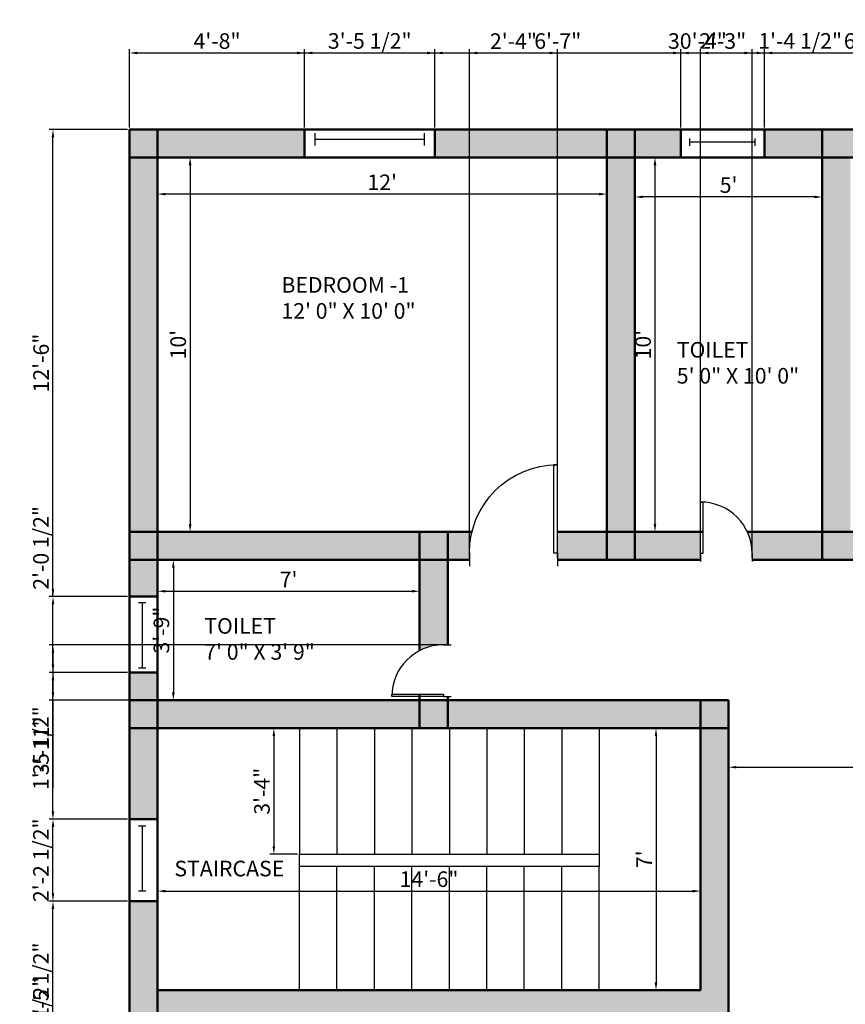
# Model space of a CAD drawing. Units: millimetres. Extents: x 2784 to 3697, y 603 to 1406.
# Tile 9 of 10: x 3272 to 3537, y 953 to 1268. Entities that reach past the tile are written whole.
import ezdxf

# ---------------------------------------------------------------- set-up
doc = ezdxf.new("R2010")
doc.units = ezdxf.units.MM
for name, color, linetype, lineweight in [('A-ANNO-DIMS', 140, 'Continuous', 18), ('A-AREA-IDEN', 150, 'Continuous', 25), ('A-DOOR', 10, 'Continuous', 25), ('A-FLOR-STRS', 200, 'Continuous', 25), ('A-GLAZ', 30, 'Continuous', 25), ('A-WALL', 2, 'Continuous', 50), ('A-WALL-PATT', 8, 'Continuous', 13)]:
    doc.layers.add(name, color=color, linetype=linetype, lineweight=lineweight)
doc.styles.get("Standard").update_dxf_attribs({"font": 'arial.ttf'})
doc.dimstyles.new('ISO-25', dxfattribs={"dimtxt": 5, "dimasz": 2.5, "dimexe": 1.25, "dimexo": 0.625, "dimtad": 1, "dimdec": 0, "dimlunit": 3, "dimtxsty": 'Standard', "dimcen": 2.5, "dimadec": 0, "dimazin": 0, "dimtfac": 1, "dimtdec": 0, "dimtmove": 0, "dimatfit": 3, "dimfxl": 1, "dimarcsym": 0})

# ---------------------------------------------------------------- blocks, each defined once
blk = doc.blocks.new('*U2')
for p, q in [((0, 0), (0, -6)), ((40, 0), (40, -6))]:
    blk.add_line(p, q)
blk.add_lwpolyline([(0, 0), (0, 40), (1.75, 40), (1.75, 0)], close=True)
blk.add_arc((0, 0), 40, 0, 90)
blk = doc.blocks.new('*U38')
for p, q in [((0, 4), (0, 0)), ((36, 4), (36, 0)), ((0, 2), (36, 2))]:
    blk.add_line(p, q)
blk = doc.blocks.new('*D39')
at = {"layer": 'A-ANNO-DIMS', "color": 0, "lineweight": -2, "transparency": 16777216}
for p, q in [((3326.67, 1221.78), (3326.67, 1106.78)), ((3327.3, 1224.28), (3327.92, 1224.28)), ((3327.3, 1104.28), (3327.92, 1104.28))]:
    blk.add_line(p, q, dxfattribs=at)
at = {"layer": 'A-ANNO-DIMS', "color": 0, "transparency": 16777216}
for points in [[(3326.25, 1221.78), (3327.09, 1221.78), (3326.67, 1224.28)], [(3326.25, 1106.78), (3327.09, 1106.78), (3326.67, 1104.28)]]:
    blk.add_solid(points, dxfattribs=at)
at = {"layer": 'Defpoints', "color": 0, "transparency": 16777216}
for p in [(3326.67, 1224.28), (3326.67, 1104.28), (3326.67, 1104.28)]:
    blk.add_point(p, dxfattribs=at)
at = {"layer": 'A-ANNO-DIMS', "color": 0, "transparency": 16777216, "insert": (3323.49, 1164.28), "char_height": 5, "attachment_point": 5, "rotation": 90}
blk.add_mtext("10'", dxfattribs=at)
blk = doc.blocks.new('*D40')
at = {"layer": 'A-ANNO-DIMS', "color": 0, "lineweight": -2, "transparency": 16777216}
for p, q in [((3316.23, 1213.16), (3316.23, 1213.79)), ((3457.73, 1212.54), (3318.73, 1212.54)), ((3460.23, 1213.16), (3460.23, 1213.79))]:
    blk.add_line(p, q, dxfattribs=at)
at = {"layer": 'A-ANNO-DIMS', "color": 0, "transparency": 16777216}
for points in [[(3318.73, 1212.95), (3318.73, 1212.12), (3316.23, 1212.54)], [(3457.73, 1212.95), (3457.73, 1212.12), (3460.23, 1212.54)]]:
    blk.add_solid(points, dxfattribs=at)
at = {"layer": 'Defpoints', "color": 0, "transparency": 16777216}
for p in [(3316.23, 1212.54), (3316.23, 1212.54), (3460.23, 1212.54)]:
    blk.add_point(p, dxfattribs=at)
at = {"layer": 'A-ANNO-DIMS', "color": 0, "transparency": 16777216, "insert": (3388.23, 1215.67), "char_height": 5, "attachment_point": 5}
blk.add_mtext("12'", dxfattribs=at)
blk = doc.blocks.new('*D41')
at = {"layer": 'A-ANNO-DIMS', "color": 0, "lineweight": -2, "transparency": 16777216}
for p, q in [((3475.35, 1224.28), (3476.89, 1224.28)), ((3475.64, 1221.78), (3475.64, 1106.78)), ((3475.35, 1104.28), (3476.89, 1104.28))]:
    blk.add_line(p, q, dxfattribs=at)
at = {"layer": 'A-ANNO-DIMS', "color": 0, "transparency": 16777216}
for points in [[(3475.22, 1221.78), (3476.06, 1221.78), (3475.64, 1224.28)], [(3475.22, 1106.78), (3476.06, 1106.78), (3475.64, 1104.28)]]:
    blk.add_solid(points, dxfattribs=at)
at = {"layer": 'Defpoints', "color": 0, "transparency": 16777216}
for p in [(3474.73, 1224.28), (3474.73, 1104.28), (3475.64, 1104.28)]:
    blk.add_point(p, dxfattribs=at)
at = {"layer": 'A-ANNO-DIMS', "color": 0, "transparency": 16777216, "insert": (3472.46, 1164.28), "char_height": 5, "attachment_point": 5, "rotation": 90}
blk.add_mtext("10'", dxfattribs=at)
blk = doc.blocks.new('*D42')
at = {"layer": 'A-ANNO-DIMS', "color": 0, "lineweight": -2, "transparency": 16777216}
for p, q in [((3469.23, 1215.87), (3469.23, 1210.37)), ((3529.23, 1215.87), (3529.23, 1210.37)), ((3526.73, 1211.62), (3471.73, 1211.62))]:
    blk.add_line(p, q, dxfattribs=at)
at = {"layer": 'A-ANNO-DIMS', "color": 0, "transparency": 16777216}
for points in [[(3471.73, 1212.04), (3471.73, 1211.21), (3469.23, 1211.62)], [(3526.73, 1212.04), (3526.73, 1211.21), (3529.23, 1211.62)]]:
    blk.add_solid(points, dxfattribs=at)
at = {"layer": 'Defpoints', "color": 0, "transparency": 16777216}
for p in [(3469.23, 1216.49), (3529.23, 1216.49), (3469.23, 1211.62)]:
    blk.add_point(p, dxfattribs=at)
at = {"layer": 'A-ANNO-DIMS', "color": 0, "transparency": 16777216, "insert": (3499.23, 1214.79), "char_height": 5, "attachment_point": 5}
blk.add_mtext("5'", dxfattribs=at)
blk = doc.blocks.new('*D45')
at = {"layer": 'A-ANNO-DIMS', "color": 0, "lineweight": -2, "transparency": 16777216}
for p, q in [((3321.44, 1095.28), (3322.55, 1095.28)), ((3321.3, 1092.78), (3321.3, 1052.78)), ((3321.44, 1050.28), (3322.55, 1050.28))]:
    blk.add_line(p, q, dxfattribs=at)
at = {"layer": 'A-ANNO-DIMS', "color": 0, "transparency": 16777216}
for points in [[(3320.88, 1092.78), (3321.71, 1092.78), (3321.3, 1095.28)], [(3320.88, 1052.78), (3321.71, 1052.78), (3321.3, 1050.28)]]:
    blk.add_solid(points, dxfattribs=at)
at = {"layer": 'Defpoints', "color": 0, "transparency": 16777216}
for p in [(3320.81, 1095.28), (3320.81, 1050.28), (3321.3, 1050.28)]:
    blk.add_point(p, dxfattribs=at)
at = {"layer": 'A-ANNO-DIMS', "color": 0, "transparency": 16777216, "insert": (3318.12, 1072.78), "char_height": 5, "attachment_point": 5, "rotation": 90}
blk.add_mtext('3\'-9"', dxfattribs=at)
blk = doc.blocks.new('*D46')
at = {"layer": 'A-ANNO-DIMS', "color": 0, "lineweight": -2, "transparency": 16777216}
for p, q in [((3316.23, 1086.57), (3316.23, 1083.98)), ((3400.23, 1085.85), (3400.23, 1086.48)), ((3318.73, 1085.23), (3397.73, 1085.23))]:
    blk.add_line(p, q, dxfattribs=at)
at = {"layer": 'A-ANNO-DIMS', "color": 0, "transparency": 16777216}
for points in [[(3318.73, 1085.64), (3318.73, 1084.81), (3316.23, 1085.23)], [(3397.73, 1085.64), (3397.73, 1084.81), (3400.23, 1085.23)]]:
    blk.add_solid(points, dxfattribs=at)
at = {"layer": 'Defpoints', "color": 0, "transparency": 16777216}
for p in [(3316.23, 1087.2), (3400.23, 1085.23), (3400.23, 1085.23)]:
    blk.add_point(p, dxfattribs=at)
at = {"layer": 'A-ANNO-DIMS', "color": 0, "transparency": 16777216, "insert": (3358.23, 1088.35), "char_height": 5, "attachment_point": 5}
blk.add_mtext("7'", dxfattribs=at)
blk = doc.blocks.new('*D55')
at = {"layer": 'A-ANNO-DIMS', "color": 0, "lineweight": -2, "transparency": 16777216}
for p, q in [((3361.11, 1041.28), (3352.26, 1041.28)), ((3353.51, 1038.78), (3353.51, 1003.45)), ((3361.11, 1000.95), (3352.26, 1000.95))]:
    blk.add_line(p, q, dxfattribs=at)
at = {"layer": 'A-ANNO-DIMS', "color": 0, "transparency": 16777216}
for points in [[(3353.09, 1038.78), (3353.93, 1038.78), (3353.51, 1041.28)], [(3353.09, 1003.45), (3353.93, 1003.45), (3353.51, 1000.95)]]:
    blk.add_solid(points, dxfattribs=at)
at = {"layer": 'Defpoints', "color": 0, "transparency": 16777216}
for p in [(3361.74, 1041.28), (3353.51, 1000.95), (3361.74, 1000.95)]:
    blk.add_point(p, dxfattribs=at)
at = {"layer": 'A-ANNO-DIMS', "color": 0, "transparency": 16777216, "insert": (3350.33, 1021.12), "char_height": 5, "attachment_point": 5, "rotation": 90}
blk.add_mtext('3\'-4"', dxfattribs=at)
blk = doc.blocks.new('*D56')
at = {"layer": 'A-ANNO-DIMS', "color": 0, "lineweight": -2, "transparency": 16777216}
for p, q in [((3316.23, 992.49), (3316.23, 987.85)), ((3490.23, 992.49), (3490.23, 987.85)), ((3318.73, 989.1), (3487.73, 989.1))]:
    blk.add_line(p, q, dxfattribs=at)
at = {"layer": 'A-ANNO-DIMS', "color": 0, "transparency": 16777216}
for points in [[(3318.73, 989.51), (3318.73, 988.68), (3316.23, 989.1)], [(3487.73, 989.51), (3487.73, 988.68), (3490.23, 989.1)]]:
    blk.add_solid(points, dxfattribs=at)
at = {"layer": 'Defpoints', "color": 0, "transparency": 16777216}
for p in [(3316.23, 993.11), (3490.23, 993.11), (3490.23, 989.1)]:
    blk.add_point(p, dxfattribs=at)
at = {"layer": 'A-ANNO-DIMS', "color": 0, "transparency": 16777216, "insert": (3403.23, 992.28), "char_height": 5, "attachment_point": 5}
blk.add_mtext('14\'-6"', dxfattribs=at)
blk = doc.blocks.new('*D57')
at = {"layer": 'A-ANNO-DIMS', "color": 0, "lineweight": -2, "transparency": 16777216}
for p, q in [((3475.97, 1038.78), (3475.97, 959.81)), ((3476.59, 1041.28), (3477.22, 1041.28)), ((3476.59, 957.31), (3477.22, 957.31))]:
    blk.add_line(p, q, dxfattribs=at)
at = {"layer": 'A-ANNO-DIMS', "color": 0, "transparency": 16777216}
for points in [[(3475.55, 1038.78), (3476.38, 1038.78), (3475.97, 1041.28)], [(3475.55, 959.81), (3476.38, 959.81), (3475.97, 957.31)]]:
    blk.add_solid(points, dxfattribs=at)
at = {"layer": 'Defpoints', "color": 0, "transparency": 16777216}
for p in [(3475.97, 1041.28), (3475.97, 957.31), (3475.97, 957.31)]:
    blk.add_point(p, dxfattribs=at)
at = {"layer": 'A-ANNO-DIMS', "color": 0, "transparency": 16777216, "insert": (3472.84, 999.3), "char_height": 5, "attachment_point": 5, "rotation": 90}
blk.add_mtext("7'", dxfattribs=at)
blk = doc.blocks.new('*D59')
at = {"layer": 'A-ANNO-DIMS', "color": 0, "lineweight": -2, "transparency": 16777216}
for p, q in [((3499.23, 1028.23), (3499.23, 1030.07)), ((3662.23, 1028.23), (3662.23, 1030.07)), ((3501.73, 1028.82), (3659.73, 1028.82))]:
    blk.add_line(p, q, dxfattribs=at)
at = {"layer": 'A-ANNO-DIMS', "color": 0, "transparency": 16777216}
for points in [[(3501.73, 1029.23), (3501.73, 1028.4), (3499.23, 1028.82)], [(3659.73, 1029.23), (3659.73, 1028.4), (3662.23, 1028.82)]]:
    blk.add_solid(points, dxfattribs=at)
at = {"layer": 'Defpoints', "color": 0, "transparency": 16777216}
for p in [(3499.23, 1027.6), (3662.23, 1028.82), (3662.23, 1027.6)]:
    blk.add_point(p, dxfattribs=at)
at = {"layer": 'A-ANNO-DIMS', "color": 0, "transparency": 16777216, "insert": (3580.73, 1032), "char_height": 5, "attachment_point": 5}
blk.add_mtext('13\'-7"', dxfattribs=at)
blk = doc.blocks.new('*D110')
at = {"layer": 'A-ANNO-DIMS', "color": 0, "lineweight": -2, "transparency": 16777216}
for p, q in [((3307.23, 1233.91), (3307.23, 1259.03)), ((3309.73, 1257.78), (3668.73, 1257.78)), ((3671.23, 1233.91), (3671.23, 1259.03))]:
    blk.add_line(p, q, dxfattribs=at)
at = {"layer": 'A-ANNO-DIMS', "color": 0, "transparency": 16777216}
for points in [[(3309.73, 1258.2), (3309.73, 1257.36), (3307.23, 1257.78)], [(3668.73, 1258.2), (3668.73, 1257.36), (3671.23, 1257.78)]]:
    blk.add_solid(points, dxfattribs=at)
at = {"layer": 'Defpoints', "color": 0, "transparency": 16777216}
for p in [(3671.23, 1257.78), (3307.23, 1233.28), (3671.23, 1233.28)]:
    blk.add_point(p, dxfattribs=at)
at = {"layer": 'A-ANNO-DIMS', "color": 0, "transparency": 16777216, "insert": (3489.23, 1260.96), "char_height": 5, "attachment_point": 5}
blk.add_mtext('30\'-4"', dxfattribs=at)
blk = doc.blocks.new('*D111')
at = {"layer": 'A-ANNO-DIMS', "color": 0, "lineweight": -2, "transparency": 16777216}
for p, q in [((3307.23, 1233.91), (3307.23, 1259.03)), ((3309.73, 1257.78), (3360.87, 1257.78)), ((3363.37, 1233.91), (3363.37, 1259.03))]:
    blk.add_line(p, q, dxfattribs=at)
at = {"layer": 'A-ANNO-DIMS', "color": 0, "transparency": 16777216}
for points in [[(3309.73, 1258.2), (3309.73, 1257.36), (3307.23, 1257.78)], [(3360.87, 1258.2), (3360.87, 1257.36), (3363.37, 1257.78)]]:
    blk.add_solid(points, dxfattribs=at)
at = {"layer": 'Defpoints', "color": 0, "transparency": 16777216}
for p in [(3363.37, 1257.78), (3307.23, 1233.28), (3363.37, 1233.28)]:
    blk.add_point(p, dxfattribs=at)
at = {"layer": 'A-ANNO-DIMS', "color": 0, "transparency": 16777216, "insert": (3335.3, 1260.96), "char_height": 5, "attachment_point": 5}
blk.add_mtext('4\'-8"', dxfattribs=at)
blk = doc.blocks.new('*D112')
at = {"layer": 'A-ANNO-DIMS', "color": 0, "lineweight": -2, "transparency": 16777216}
for p, q in [((3363.37, 1233.91), (3363.37, 1259.03)), ((3365.87, 1257.78), (3402.6, 1257.78)), ((3405.1, 1233.91), (3405.1, 1259.03))]:
    blk.add_line(p, q, dxfattribs=at)
at = {"layer": 'A-ANNO-DIMS', "color": 0, "transparency": 16777216}
for points in [[(3365.87, 1258.2), (3365.87, 1257.36), (3363.37, 1257.78)], [(3402.6, 1258.2), (3402.6, 1257.36), (3405.1, 1257.78)]]:
    blk.add_solid(points, dxfattribs=at)
at = {"layer": 'Defpoints', "color": 0, "transparency": 16777216}
for p in [(3405.1, 1257.78), (3363.37, 1233.28), (3405.1, 1233.28)]:
    blk.add_point(p, dxfattribs=at)
at = {"layer": 'A-ANNO-DIMS', "color": 0, "transparency": 16777216, "insert": (3384.23, 1260.99), "char_height": 5, "attachment_point": 5}
blk.add_mtext('3\'-5 1/2"', dxfattribs=at)
blk = doc.blocks.new('*D113')
at = {"layer": 'A-ANNO-DIMS', "color": 0, "lineweight": -2, "transparency": 16777216}
for p, q in [((3405.1, 1233.91), (3405.1, 1259.03)), ((3407.6, 1257.78), (3481.39, 1257.78)), ((3483.89, 1233.91), (3483.89, 1259.03))]:
    blk.add_line(p, q, dxfattribs=at)
at = {"layer": 'A-ANNO-DIMS', "color": 0, "transparency": 16777216}
for points in [[(3407.6, 1258.2), (3407.6, 1257.36), (3405.1, 1257.78)], [(3481.39, 1258.2), (3481.39, 1257.36), (3483.89, 1257.78)]]:
    blk.add_solid(points, dxfattribs=at)
at = {"layer": 'Defpoints', "color": 0, "transparency": 16777216}
for p in [(3483.89, 1257.78), (3405.1, 1233.28), (3483.89, 1233.28)]:
    blk.add_point(p, dxfattribs=at)
at = {"layer": 'A-ANNO-DIMS', "color": 0, "transparency": 16777216, "insert": (3444.49, 1260.96), "char_height": 5, "attachment_point": 5}
blk.add_mtext('6\'-7"', dxfattribs=at)
blk = doc.blocks.new('*D114')
at = {"layer": 'A-ANNO-DIMS', "color": 0, "lineweight": -2, "transparency": 16777216}
for p, q in [((3483.89, 1233.91), (3483.89, 1259.03)), ((3486.39, 1257.78), (3508.27, 1257.78)), ((3510.77, 1233.91), (3510.77, 1259.03))]:
    blk.add_line(p, q, dxfattribs=at)
at = {"layer": 'A-ANNO-DIMS', "color": 0, "transparency": 16777216}
for points in [[(3486.39, 1258.2), (3486.39, 1257.36), (3483.89, 1257.78)], [(3508.27, 1258.2), (3508.27, 1257.36), (3510.77, 1257.78)]]:
    blk.add_solid(points, dxfattribs=at)
at = {"layer": 'Defpoints', "color": 0, "transparency": 16777216}
for p in [(3510.77, 1257.78), (3483.89, 1233.28), (3510.77, 1233.28)]:
    blk.add_point(p, dxfattribs=at)
at = {"layer": 'A-ANNO-DIMS', "color": 0, "transparency": 16777216, "insert": (3497.33, 1260.96), "char_height": 5, "attachment_point": 5}
blk.add_mtext('2\'-3"', dxfattribs=at)
blk = doc.blocks.new('*D115')
at = {"layer": 'A-ANNO-DIMS', "color": 0, "lineweight": -2, "transparency": 16777216}
for p, q in [((3510.77, 1233.91), (3510.77, 1259.03)), ((3513.27, 1257.78), (3585.87, 1257.78)), ((3588.37, 1233.91), (3588.37, 1259.03))]:
    blk.add_line(p, q, dxfattribs=at)
at = {"layer": 'A-ANNO-DIMS', "color": 0, "transparency": 16777216}
for points in [[(3513.27, 1258.2), (3513.27, 1257.36), (3510.77, 1257.78)], [(3585.87, 1258.2), (3585.87, 1257.36), (3588.37, 1257.78)]]:
    blk.add_solid(points, dxfattribs=at)
at = {"layer": 'Defpoints', "color": 0, "transparency": 16777216}
for p in [(3588.37, 1257.78), (3510.77, 1233.28), (3588.37, 1233.28)]:
    blk.add_point(p, dxfattribs=at)
at = {"layer": 'A-ANNO-DIMS', "color": 0, "transparency": 16777216, "insert": (3549.57, 1260.99), "char_height": 5, "attachment_point": 5}
blk.add_mtext('6\'-5 1/2"', dxfattribs=at)
blk = doc.blocks.new('*D124')
at = {"layer": 'A-ANNO-DIMS', "color": 0, "lineweight": -2, "transparency": 16777216}
for p, q in [((3282.73, 932.57), (3282.73, 961.35)), ((3306.6, 932.57), (3281.48, 932.57)), ((3282.73, 910.67), (3282.73, 930.07)), ((3306.6, 908.17), (3281.48, 908.17))]:
    blk.add_line(p, q, dxfattribs=at)
at = {"layer": 'A-ANNO-DIMS', "color": 0, "transparency": 16777216}
for points in [[(3282.31, 930.07), (3283.14, 930.07), (3282.73, 932.57)], [(3282.31, 910.67), (3283.14, 910.67), (3282.73, 908.17)]]:
    blk.add_solid(points, dxfattribs=at)
at = {"layer": 'Defpoints', "color": 0, "transparency": 16777216}
for p in [(3282.73, 932.57), (3307.23, 932.57), (3307.23, 908.17)]:
    blk.add_point(p, dxfattribs=at)
at = {"layer": 'A-ANNO-DIMS', "color": 0, "transparency": 16777216, "insert": (3279.52, 948.21), "char_height": 5, "attachment_point": 5, "rotation": 90}
blk.add_mtext('2\'-0 1/2"', dxfattribs=at)
blk = doc.blocks.new('*D125')
at = {"layer": 'A-ANNO-DIMS', "color": 0, "lineweight": -2, "transparency": 16777216}
for p, q in [((3306.6, 985.84), (3281.48, 985.84)), ((3282.73, 935.07), (3282.73, 983.34)), ((3306.6, 932.57), (3281.48, 932.57))]:
    blk.add_line(p, q, dxfattribs=at)
at = {"layer": 'A-ANNO-DIMS', "color": 0, "transparency": 16777216}
for points in [[(3282.31, 983.34), (3283.14, 983.34), (3282.73, 985.84)], [(3282.31, 935.07), (3283.14, 935.07), (3282.73, 932.57)]]:
    blk.add_solid(points, dxfattribs=at)
at = {"layer": 'Defpoints', "color": 0, "transparency": 16777216}
for p in [(3282.73, 985.84), (3307.23, 985.84), (3307.23, 932.57)]:
    blk.add_point(p, dxfattribs=at)
at = {"layer": 'A-ANNO-DIMS', "color": 0, "transparency": 16777216, "insert": (3279.52, 959.21), "char_height": 5, "attachment_point": 5, "rotation": 90}
blk.add_mtext('4\'-5 1/2"', dxfattribs=at)
blk = doc.blocks.new('*D126')
at = {"layer": 'A-ANNO-DIMS', "color": 0, "lineweight": -2, "transparency": 16777216}
for p, q in [((3306.6, 1012.14), (3281.48, 1012.14)), ((3282.73, 988.34), (3282.73, 1009.64)), ((3306.6, 985.84), (3281.48, 985.84))]:
    blk.add_line(p, q, dxfattribs=at)
at = {"layer": 'A-ANNO-DIMS', "color": 0, "transparency": 16777216}
for points in [[(3282.31, 1009.64), (3283.14, 1009.64), (3282.73, 1012.14)], [(3282.31, 988.34), (3283.14, 988.34), (3282.73, 985.84)]]:
    blk.add_solid(points, dxfattribs=at)
at = {"layer": 'Defpoints', "color": 0, "transparency": 16777216}
for p in [(3282.73, 1012.14), (3307.23, 1012.14), (3307.23, 985.84)]:
    blk.add_point(p, dxfattribs=at)
at = {"layer": 'A-ANNO-DIMS', "color": 0, "transparency": 16777216, "insert": (3279.52, 998.99), "char_height": 5, "attachment_point": 5, "rotation": 90}
blk.add_mtext('2\'-2 1/2"', dxfattribs=at)
blk = doc.blocks.new('*D127')
at = {"layer": 'A-ANNO-DIMS', "color": 0, "lineweight": -2, "transparency": 16777216}
for p, q in [((3306.6, 1059.19), (3281.48, 1059.19)), ((3282.73, 1014.64), (3282.73, 1056.69)), ((3306.6, 1012.14), (3281.48, 1012.14))]:
    blk.add_line(p, q, dxfattribs=at)
at = {"layer": 'A-ANNO-DIMS', "color": 0, "transparency": 16777216}
for points in [[(3282.31, 1056.69), (3283.14, 1056.69), (3282.73, 1059.19)], [(3282.31, 1014.64), (3283.14, 1014.64), (3282.73, 1012.14)]]:
    blk.add_solid(points, dxfattribs=at)
at = {"layer": 'Defpoints', "color": 0, "transparency": 16777216}
for p in [(3282.73, 1059.19), (3307.23, 1059.19), (3307.23, 1012.14)]:
    blk.add_point(p, dxfattribs=at)
at = {"layer": 'A-ANNO-DIMS', "color": 0, "transparency": 16777216, "insert": (3279.55, 1035.67), "char_height": 5, "attachment_point": 5, "rotation": 90}
blk.add_mtext('3\'-11"', dxfattribs=at)
blk = doc.blocks.new('*D128')
at = {"layer": 'A-ANNO-DIMS', "color": 0, "lineweight": -2, "transparency": 16777216}
for p, q in [((3282.73, 1083.49), (3282.73, 1112.27)), ((3306.6, 1083.49), (3281.48, 1083.49)), ((3282.73, 1061.69), (3282.73, 1080.99)), ((3306.6, 1059.19), (3281.48, 1059.19))]:
    blk.add_line(p, q, dxfattribs=at)
at = {"layer": 'A-ANNO-DIMS', "color": 0, "transparency": 16777216}
for points in [[(3282.31, 1080.99), (3283.14, 1080.99), (3282.73, 1083.49)], [(3282.31, 1061.69), (3283.14, 1061.69), (3282.73, 1059.19)]]:
    blk.add_solid(points, dxfattribs=at)
at = {"layer": 'Defpoints', "color": 0, "transparency": 16777216}
for p in [(3282.73, 1083.49), (3307.23, 1083.49), (3307.23, 1059.19)]:
    blk.add_point(p, dxfattribs=at)
at = {"layer": 'A-ANNO-DIMS', "color": 0, "transparency": 16777216, "insert": (3279.52, 1099.13), "char_height": 5, "attachment_point": 5, "rotation": 90}
blk.add_mtext('2\'-0 1/2"', dxfattribs=at)
blk = doc.blocks.new('*D129')
at = {"layer": 'A-ANNO-DIMS', "color": 0, "lineweight": -2, "transparency": 16777216}
for p, q in [((3306.6, 1233.28), (3281.48, 1233.28)), ((3282.73, 1085.99), (3282.73, 1230.78)), ((3306.6, 1083.49), (3281.48, 1083.49))]:
    blk.add_line(p, q, dxfattribs=at)
at = {"layer": 'A-ANNO-DIMS', "color": 0, "transparency": 16777216}
for points in [[(3282.31, 1230.78), (3283.14, 1230.78), (3282.73, 1233.28)], [(3282.31, 1085.99), (3283.14, 1085.99), (3282.73, 1083.49)]]:
    blk.add_solid(points, dxfattribs=at)
at = {"layer": 'Defpoints', "color": 0, "transparency": 16777216}
for p in [(3282.73, 1233.28), (3307.23, 1233.28), (3307.23, 1083.49)]:
    blk.add_point(p, dxfattribs=at)
at = {"layer": 'A-ANNO-DIMS', "color": 0, "transparency": 16777216, "insert": (3279.55, 1158.39), "char_height": 5, "attachment_point": 5, "rotation": 90}
blk.add_mtext('12\'-6"', dxfattribs=at)
blk = doc.blocks.new('*D132')
at = {"layer": 'A-ANNO-DIMS', "color": 0, "lineweight": -2, "transparency": 16777216}
for p, q in [((3416.17, 1095.91), (3416.17, 1259.03)), ((3418.67, 1257.78), (3441.89, 1257.78)), ((3444.39, 1095.91), (3444.39, 1259.03))]:
    blk.add_line(p, q, dxfattribs=at)
at = {"layer": 'A-ANNO-DIMS', "color": 0, "transparency": 16777216}
for points in [[(3418.67, 1258.2), (3418.67, 1257.36), (3416.17, 1257.78)], [(3441.89, 1258.2), (3441.89, 1257.36), (3444.39, 1257.78)]]:
    blk.add_solid(points, dxfattribs=at)
at = {"layer": 'Defpoints', "color": 0, "transparency": 16777216}
for p in [(3444.39, 1257.78), (3416.17, 1095.28), (3444.39, 1095.28)]:
    blk.add_point(p, dxfattribs=at)
at = {"layer": 'A-ANNO-DIMS', "color": 0, "transparency": 16777216, "insert": (3430.28, 1260.92), "char_height": 5, "attachment_point": 5}
blk.add_mtext('2\'-4"', dxfattribs=at)
blk = doc.blocks.new('*D133')
at = {"layer": 'A-ANNO-DIMS', "color": 0, "lineweight": -2, "transparency": 16777216}
for p, q in [((3490.27, 1095.91), (3490.27, 1259.03)), ((3492.77, 1257.78), (3504.3, 1257.78)), ((3506.8, 1095.91), (3506.8, 1259.03)), ((3506.8, 1257.78), (3535.02, 1257.78))]:
    blk.add_line(p, q, dxfattribs=at)
at = {"layer": 'A-ANNO-DIMS', "color": 0, "transparency": 16777216}
for points in [[(3492.77, 1258.2), (3492.77, 1257.36), (3490.27, 1257.78)], [(3504.3, 1258.2), (3504.3, 1257.36), (3506.8, 1257.78)]]:
    blk.add_solid(points, dxfattribs=at)
at = {"layer": 'Defpoints', "color": 0, "transparency": 16777216}
for p in [(3506.8, 1257.78), (3490.27, 1095.28), (3506.8, 1095.28)]:
    blk.add_point(p, dxfattribs=at)
at = {"layer": 'A-ANNO-DIMS', "color": 0, "transparency": 16777216, "insert": (3522.16, 1260.99), "char_height": 5, "attachment_point": 5}
blk.add_mtext('1\'-4 1/2"', dxfattribs=at)
blk = doc.blocks.new('*D135')
at = {"layer": 'A-ANNO-DIMS', "color": 0, "lineweight": -2, "transparency": 16777216}
for p, q in [((3408.6, 1068.02), (3281.48, 1068.02)), ((3282.73, 1065.52), (3282.73, 1052.78)), ((3408.6, 1050.28), (3281.48, 1050.28)), ((3282.73, 1050.28), (3282.73, 1022.06))]:
    blk.add_line(p, q, dxfattribs=at)
at = {"layer": 'A-ANNO-DIMS', "color": 0, "transparency": 16777216}
for points in [[(3282.31, 1065.52), (3283.14, 1065.52), (3282.73, 1068.02)], [(3282.31, 1052.78), (3283.14, 1052.78), (3282.73, 1050.28)]]:
    blk.add_solid(points, dxfattribs=at)
at = {"layer": 'Defpoints', "color": 0, "transparency": 16777216}
for p in [(3409.23, 1068.02), (3282.73, 1050.28), (3409.23, 1050.28)]:
    blk.add_point(p, dxfattribs=at)
at = {"layer": 'A-ANNO-DIMS', "color": 0, "transparency": 16777216, "insert": (3279.52, 1034.92), "char_height": 5, "attachment_point": 5, "rotation": 90}
blk.add_mtext('1\'-5 1/2"', dxfattribs=at)

msp = doc.modelspace()

# ---------------------------------------------------------------- hatches: boundary and pattern name
at = {"layer": 'A-WALL-PATT'}
h = msp.add_hatch(color=256, dxfattribs=at)
h.dxf.hatch_style = 1
h.paths.add_polyline_path([(3316.23, 1224.28), (3307.23, 1224.28), (3307.23, 1104.28), (3316.23, 1104.28)])
h.paths.add_polyline_path([(3316.23, 1233.28), (3307.23, 1233.28), (3307.23, 1224.28), (3316.23, 1224.28)])
h.paths.add_polyline_path([(3363.37, 1233.28), (3316.23, 1233.28), (3316.23, 1224.28), (3363.37, 1224.28)])
h.paths.add_polyline_path([(3460.23, 1233.28), (3405.1, 1233.28), (3405.1, 1224.28), (3460.23, 1224.28)])
h.paths.add_polyline_path([(3469.23, 1233.28), (3460.23, 1233.28), (3460.23, 1224.28), (3469.23, 1224.28)])
h.paths.add_polyline_path([(3469.23, 1224.28), (3460.23, 1224.28), (3460.23, 1104.28), (3469.23, 1104.28)])
h.paths.add_polyline_path([(3469.23, 1104.28), (3460.23, 1104.28), (3460.23, 1095.28), (3469.23, 1095.28)])
h.paths.add_polyline_path([(3460.23, 1104.28), (3444.39, 1104.28), (3444.39, 1097.52), (3444.39, 1095.28), (3460.23, 1095.28)])
h.paths.add_polyline_path([(3409.23, 1095.28), (3400.23, 1095.28), (3400.23, 1066.17, -0.119943), (3407.82, 1068.02), (3409.23, 1068.02)])
h.paths.add_polyline_path([(3409.23, 1104.28), (3400.23, 1104.28), (3400.23, 1095.28), (3409.23, 1095.28)])
h.paths.add_polyline_path([(3400.23, 1104.28), (3316.23, 1104.28), (3316.23, 1095.28), (3400.23, 1095.28)])
h.paths.add_polyline_path([(3316.23, 1104.28), (3307.23, 1104.28), (3307.23, 1095.28), (3316.23, 1095.28)])
h.paths.add_polyline_path([(3316.23, 1095.28), (3307.23, 1095.28), (3307.23, 1083.49), (3316.23, 1083.49)])
h.paths.add_polyline_path([(3416.17, 1097.52, -0.060509), (3416.99, 1104.28), (3409.23, 1104.28), (3409.23, 1095.28), (3416.17, 1095.28)])
h.paths.add_polyline_path([(3538.23, 1224.28), (3529.23, 1224.28), (3529.23, 1104.28), (3538.23, 1104.28)])
h.paths.add_polyline_path([(3538.23, 1233.28), (3529.23, 1233.28), (3529.23, 1224.28), (3538.23, 1224.28)])
h.paths.add_polyline_path([(3529.23, 1233.28), (3510.77, 1233.28), (3510.77, 1224.28), (3529.23, 1224.28)])
h.paths.add_polyline_path([(3483.89, 1233.28), (3469.23, 1233.28), (3469.23, 1224.28), (3483.89, 1224.28)])
h.paths.add_polyline_path([(3662.23, 1233.28), (3629.82, 1233.28), (3629.82, 1224.28), (3662.23, 1224.28)])
h.paths.add_polyline_path([(3671.23, 1233.28), (3662.23, 1233.28), (3662.23, 1224.28), (3671.23, 1224.28)])
h.paths.add_polyline_path([(3671.23, 1224.28), (3662.23, 1224.28), (3662.23, 1104.28), (3671.23, 1104.28)])
h.paths.add_polyline_path([(3588.37, 1233.28), (3538.23, 1233.28), (3538.23, 1224.28), (3588.37, 1224.28)])
h.paths.add_polyline_path([(3662.23, 1104.28), (3579.01, 1104.28, -0.053945), (3579.66, 1098.24), (3579.66, 1095.28), (3662.23, 1095.28)])
h.paths.add_polyline_path([(3671.23, 1104.28), (3662.23, 1104.28), (3662.23, 1095.28), (3671.23, 1095.28)])
h.paths.add_polyline_path([(3551.44, 1104.28), (3538.23, 1104.28), (3538.23, 1095.28), (3551.44, 1095.28), (3551.44, 1098.24)])
h.paths.add_polyline_path([(3538.23, 1104.28), (3529.23, 1104.28), (3529.23, 1095.28), (3538.23, 1095.28)])
h.paths.add_polyline_path([(3671.23, 1095.28), (3662.23, 1095.28), (3662.23, 903.31), (3671.23, 903.31)])
h.paths.add_polyline_path([(3316.23, 985.84), (3307.23, 985.84), (3307.23, 932.57), (3316.23, 932.57)])
h.paths.add_polyline_path([(3316.23, 1041.28), (3307.23, 1041.28), (3307.23, 1012.14), (3316.23, 1012.14)])
h.paths.add_polyline_path([(3316.23, 1050.28), (3307.23, 1050.28), (3307.23, 1041.28), (3316.23, 1041.28)])
h.paths.add_polyline_path([(3400.23, 1050.28), (3316.23, 1050.28), (3316.23, 1041.28), (3400.23, 1041.28)])
h.paths.add_polyline_path([(3316.23, 1059.19), (3307.23, 1059.19), (3307.23, 1050.28), (3316.23, 1050.28)])
h.paths.add_polyline_path([(3316.23, 908.17), (3307.23, 908.17), (3307.23, 774.31), (3316.23, 774.31)])
h.paths.add_polyline_path([(3316.23, 774.31), (3307.23, 774.31), (3307.23, 765.31), (3316.23, 765.31)])
h.paths.add_polyline_path([(3372.55, 774.31), (3316.23, 774.31), (3316.23, 765.31), (3372.55, 765.31)])
h.paths.add_polyline_path([(3505.23, 774.31), (3416.56, 774.31), (3416.56, 765.31), (3505.23, 765.31)])
h.paths.add_polyline_path([(3568.83, 774.31), (3514.23, 774.31), (3514.23, 765.31), (3568.83, 765.31)])
h.paths.add_polyline_path([(3514.23, 774.31), (3505.23, 774.31), (3505.23, 765.31), (3514.23, 765.31)])
h.paths.add_polyline_path([(3514.23, 894.31), (3505.23, 894.31), (3505.23, 774.31), (3514.23, 774.31)])
h.paths.add_polyline_path([(3514.23, 903.31), (3505.23, 903.31), (3505.23, 894.31), (3514.23, 894.31)])
h.paths.add_polyline_path([(3473.23, 948.31), (3464.23, 948.31), (3464.23, 903.31), (3473.23, 903.31)])
h.paths.add_polyline_path([(3473.23, 903.31), (3464.23, 903.31), (3464.23, 894.31), (3473.23, 894.31)])
h.paths.add_polyline_path([(3464.23, 903.31), (3421.03, 903.31, -0.144956), (3423.7, 894.31), (3464.23, 894.31)])
h.paths.add_polyline_path([(3385.23, 903.31), (3376.23, 903.31), (3376.23, 894.31), (3385.23, 894.31)])
h.paths.add_polyline_path([(3385.23, 948.31), (3376.23, 948.31), (3376.23, 903.31), (3385.23, 903.31)])
h.paths.add_polyline_path([(3407.17, 903.31), (3385.23, 903.31), (3385.23, 894.31), (3407.17, 894.31)])
h.paths.add_polyline_path([(3353.12, 903.31), (3316.23, 903.31), (3316.23, 894.31), (3353.12, 894.31), (3353.12, 895.49)])
h.paths.add_polyline_path([(3376.23, 903.31), (3367.68, 903.31, -0.123903), (3369.65, 895.49), (3369.65, 894.31), (3376.23, 894.31)])
h.paths.add_polyline_path([(3499.23, 957.31), (3499.23, 1041.28), (3490.23, 1041.28), (3490.23, 957.31), (3316.23, 957.31), (3316.23, 948.31), (3490.23, 948.31), (3499.23, 948.31)])
h.paths.add_polyline_path([(3490.23, 1050.28), (3485.56, 1050.28), (3409.23, 1050.28), (3409.23, 1041.28), (3490.23, 1041.28)])
h.paths.add_polyline_path([(3409.23, 1050.28), (3400.23, 1050.28), (3400.23, 1041.28), (3409.23, 1041.28)])
h.paths.add_polyline_path([(3499.23, 1050.28), (3490.23, 1050.28), (3490.23, 1041.28), (3499.23, 1041.28)])
h.paths.add_polyline_path([(3671.23, 894.31), (3662.23, 894.31), (3662.23, 774.31), (3671.23, 774.31)])
h.paths.add_polyline_path([(3671.23, 903.31), (3662.23, 903.31), (3662.23, 894.31), (3671.23, 894.31)])
h.paths.add_polyline_path([(3662.23, 903.31), (3558.05, 903.31, -0.082354), (3555.98, 894.31), (3662.23, 894.31)])
h.paths.add_polyline_path([(3529.88, 903.31), (3514.23, 903.31), (3514.23, 894.31), (3529.88, 894.31)])
h.paths.add_polyline_path([(3531.12, 903.31), (3529.88, 903.31), (3529.88, 894.31), (3531.12, 894.31)])
h.paths.add_polyline_path([(3662.23, 774.31), (3610.06, 774.31), (3610.06, 765.31), (3662.23, 765.31)])
h.paths.add_polyline_path([(3671.23, 774.31), (3662.23, 774.31), (3662.23, 765.31), (3671.23, 765.31)])
h.paths.add_polyline_path([(3544.99, 801.01), (3590.84, 801.01), (3590.84, 819.67), (3544.99, 819.67)], flags=9)
h.paths.add_polyline_path([(3347.99, 824.43), (3394.58, 824.43), (3394.58, 843.09), (3347.99, 843.09)], flags=9)
h.paths.add_polyline_path([(3546.35, 988.53), (3592.21, 988.53), (3592.21, 1007.19), (3546.35, 1007.19)], flags=9)
h.paths.add_polyline_path([(3329.63, 1060.44), (3367.72, 1060.44), (3367.72, 1079.1), (3329.63, 1079.1)], flags=9)
h.paths.add_polyline_path([(3353.92, 1169.75), (3400.92, 1169.75), (3400.92, 1188.4), (3353.92, 1188.4)], flags=9)
h = msp.add_hatch(color=256, dxfattribs=at)
h.dxf.hatch_style = 1
h.paths.add_polyline_path([(3490.27, 1104.28), (3469.23, 1104.28), (3469.23, 1095.28), (3490.27, 1095.28), (3490.27, 1097.29)])
h.paths.add_polyline_path([(3529.23, 1104.28), (3505.25, 1104.28, -0.109612), (3506.8, 1097.29), (3506.8, 1095.28), (3529.23, 1095.28)])

# ---------------------------------------------------------------- linework, layer by layer
at = {"layer": 'A-FLOR-STRS'}
for p, q in [((3361.74, 1041.28), (3361.74, 1000.95)), ((3373.74, 1041.28), (3373.74, 1000.95)), ((3385.74, 1041.28), (3385.74, 1000.95)), ((3397.74, 1041.28), (3397.74, 1000.95)), ((3409.74, 1041.28), (3409.74, 1000.95)), ((3421.74, 1041.28), (3421.74, 1000.95)), ((3433.74, 1041.28), (3433.74, 1000.95)), ((3445.74, 1041.28), (3445.74, 1000.95)), ((3457.74, 1041.28), (3457.74, 1000.95)), ((3361.74, 1000.95), (3457.74, 1000.95)), ((3361.74, 997.03), (3361.74, 1000.95)), ((3361.74, 1000.95), (3457.74, 1000.95)), ((3457.74, 1000.95), (3457.74, 997.03)), ((3361.74, 957.31), (3361.74, 997.03)), ((3457.74, 997.03), (3361.74, 997.03)), ((3373.74, 957.31), (3373.74, 997.03)), ((3385.74, 957.31), (3385.74, 997.03)), ((3397.74, 957.31), (3397.74, 997.03)), ((3409.74, 957.31), (3409.74, 997.03)), ((3421.74, 957.31), (3421.74, 997.03)), ((3433.74, 957.31), (3433.74, 997.03)), ((3445.74, 957.31), (3445.74, 997.03)), ((3457.74, 957.31), (3457.74, 997.03)), ((3354.86, 957.31), (3316.23, 957.31))]:
    msp.add_line(p, q, dxfattribs=at)
at = {"layer": 'A-WALL'}
for p, q in [((3307.23, 1233.28), (3307.23, 765.31)), ((3307.23, 1233.28), (3671.23, 1233.28)), ((3316.23, 1233.28), (3316.23, 765.31)), ((3363.37, 1233.28), (3363.37, 1224.28)), ((3405.1, 1233.28), (3405.1, 1224.28)), ((3460.23, 1233.28), (3460.23, 1095.28)), ((3469.23, 1233.28), (3469.23, 1095.28)), ((3483.89, 1233.28), (3483.89, 1224.28)), ((3510.77, 1233.28), (3510.77, 1224.28)), ((3529.23, 1233.28), (3529.23, 1095.28)), ((3307.23, 1224.28), (3671.23, 1224.28)), ((3307.23, 1104.28), (3416.99, 1104.28)), ((3400.23, 1104.28), (3400.23, 1066.17)), ((3409.23, 1104.28), (3409.23, 1068.02)), ((3444.39, 1104.28), (3490.99, 1104.28)), ((3505.25, 1104.28), (3552.67, 1104.28)), ((3307.23, 1095.28), (3416.17, 1095.28)), ((3444.39, 1095.28), (3490.27, 1095.28)), ((3506.8, 1095.28), (3551.44, 1095.28)), ((3316.23, 1083.49), (3307.23, 1083.49)), ((3316.23, 1059.19), (3307.23, 1059.19)), ((3400.23, 1052.22), (3400.23, 1041.28)), ((3409.23, 1051.49), (3409.23, 1041.28)), ((3307.23, 1050.28), (3409.23, 1050.28)), ((3409.23, 1050.28), (3490.23, 1050.28)), ((3485.56, 1050.28), (3499.23, 1050.28)), ((3490.23, 957.31), (3490.23, 1050.28)), ((3499.23, 957.31), (3499.23, 1050.28)), ((3307.23, 1041.28), (3409.23, 1041.28)), ((3409.23, 1041.28), (3499.23, 1041.28)), ((3316.23, 1012.14), (3307.23, 1012.14)), ((3316.23, 985.84), (3307.23, 985.84)), ((3316.23, 957.31), (3490.23, 957.31)), ((3499.23, 948.31), (3499.23, 957.31))]:
    msp.add_line(p, q, dxfattribs=at)

# ---------------------------------------------------------------- block references
at = {"layer": 'A-DOOR'}
for p, xscale, yscale, zscale in [((3444.39, 1097.52), -0.7055841571326333, 0.7055841571326333, 0.7055841571326333), ((3490.27, 1097.29), 0.413209421180039, 0.413209421180039, 0.413209421180039)]:
    msp.add_blockref('*U2', p, dxfattribs=dict(at, xscale=xscale, yscale=yscale, zscale=zscale))
at = {"layer": 'A-DOOR', "xscale": 0.413209421180039, "yscale": 0.413209421180039, "zscale": 0.413209421180039, "rotation": 90}
msp.add_blockref('*U2', (3407.82, 1051.49), dxfattribs=at)
at = {"layer": 'A-GLAZ', "xscale": 0.9748873049904094, "yscale": 0.9748873049904094, "zscale": 0.9748873049904094}
msp.add_blockref('*U38', (3366.59, 1228.17), dxfattribs=at)
msp.add_blockref('*U38', (3366.59, 1228.17), dxfattribs=at)
at = {"layer": 'A-GLAZ', "xscale": 0.5811470115210491, "yscale": 0.5811470115210491, "zscale": 0.5811470115210491}
for p, rotation in [((3507.71, 1230.35), 180), ((3310.15, 1081.46), 269.9999999999999), ((3310.15, 1009.97), 269.9999999999999)]:
    msp.add_blockref('*U38', p, dxfattribs=dict(at, rotation=rotation))

# ---------------------------------------------------------------- texts
at = {"layer": 'A-AREA-IDEN', "char_height": 5, "attachment_point": 1}
for s, width, insert in [('BEDROOM -1 \\P12\' 0" X 10\' 0"', 77.1579, (3355.93, 1185.92)), ('TOILET\\P5\' 0" X 10\' 0"', 41.3019, (3482.63, 1165.13)), ('TOILET \\P7\' 0" X 3\' 9"', 45.1307, (3331.21, 1076.61)), ('STAIRCASE', 28.4176, (3321.63, 998.83))]:
    msp.add_mtext_dynamic_manual_height_columns(s, width=width, gutter_width=12.5, heights=[0], dxfattribs=dict(at, insert=insert))

# ---------------------------------------------------------------- dimensions: what is measured, and where the dimension line sits
at = {"layer": 'A-ANNO-DIMS'}
for base, p1, p2, override, picture, middle in [((3405.1, 1257.78), (3363.37, 1233.28), (3405.1, 1233.28), {"dimdec": 1, "dimlfac": 1, "dimrnd": 0, "dimzin": 1, "dimdsep": 46, "dimlunit": 4, "dimfrac": 2}, '*D112', (3384.23, 1260.99)), ((3506.8, 1257.78), (3490.27, 1095.28), (3506.8, 1095.28), {"dimdec": 1, "dimlfac": 1, "dimrnd": 0, "dimzin": 1, "dimdsep": 46, "dimlunit": 4, "dimfrac": 2}, '*D133', (3522.16, 1260.99)), ((3588.37, 1257.78), (3510.77, 1233.28), (3588.37, 1233.28), {"dimdec": 1, "dimlfac": 1, "dimrnd": 0, "dimzin": 1, "dimdsep": 46, "dimlunit": 4, "dimfrac": 2}, '*D115', (3549.57, 1260.99)), ((3671.23, 1257.78), (3307.23, 1233.28), (3671.23, 1233.28), {"dimdec": 1, "dimlfac": 1, "dimrnd": 0, "dimzin": 1, "dimdsep": 46, "dimlunit": 4, "dimfrac": 2}, '*D110', (3489.23, 1260.96)), ((3363.37, 1257.78), (3307.23, 1233.28), (3363.37, 1233.28), {"dimdec": 1, "dimlfac": 1, "dimrnd": 0, "dimzin": 1, "dimdsep": 46, "dimlunit": 4, "dimfrac": 2}, '*D111', (3335.3, 1260.96)), ((3483.89, 1257.78), (3405.1, 1233.28), (3483.89, 1233.28), {"dimdec": 1, "dimlfac": 1, "dimrnd": 0, "dimzin": 1, "dimdsep": 46, "dimlunit": 4, "dimfrac": 2}, '*D113', (3444.49, 1260.96)), ((3444.39, 1257.78), (3416.17, 1095.28), (3444.39, 1095.28), {"dimdec": 1, "dimlfac": 1, "dimrnd": 0, "dimzin": 1, "dimdsep": 46, "dimlunit": 4, "dimfrac": 2}, '*D132', (3430.28, 1260.92)), ((3510.77, 1257.78), (3483.89, 1233.28), (3510.77, 1233.28), {"dimdec": 1, "dimlfac": 1, "dimrnd": 0, "dimzin": 1, "dimdsep": 46, "dimlunit": 4, "dimfrac": 2}, '*D114', (3497.33, 1260.96)), ((3316.23, 1212.54), (3460.23, 1212.54), (3316.23, 1212.54), {"dimclrd": 0, "dimclre": 0, "dimclrt": 0}, '*D40', (3388.23, 1215.67)), ((3469.23, 1211.62), (3529.23, 1216.49), (3469.23, 1216.49), {"dimclrd": 0, "dimclre": 0, "dimclrt": 0}, '*D42', (3499.23, 1214.79)), ((3400.23, 1085.23), (3316.23, 1087.2), (3400.23, 1085.23), {"dimclrd": 0, "dimclre": 0, "dimclrt": 0}, '*D46', (3358.23, 1088.35)), ((3662.23, 1028.82), (3499.23, 1027.6), (3662.23, 1027.6), {"dimclrd": 0, "dimclre": 0, "dimclrt": 0}, '*D59', (3580.73, 1032)), ((3490.23, 989.1), (3316.23, 993.11), (3490.23, 993.11), {"dimclrd": 0, "dimclre": 0, "dimclrt": 0}, '*D56', (3403.23, 992.28))]:
    dim = msp.add_linear_dim(base=base, p1=p1, p2=p2, dimstyle='ISO-25', override=override, dxfattribs=at)
    dim.commit()
    dim.dimension.update_dxf_attribs({"geometry": picture, "text_midpoint": middle})
for base, p1, p2, override, picture, middle in [((3282.73, 1233.28), (3307.23, 1083.49), (3307.23, 1233.28), {"dimdec": 1, "dimlfac": 1, "dimrnd": 0, "dimzin": 1, "dimdsep": 46, "dimlunit": 4, "dimfrac": 2}, '*D129', (3279.55, 1158.39)), ((3326.67, 1104.28), (3326.67, 1224.28), (3326.67, 1104.28), {"dimclrd": 0, "dimclre": 0, "dimclrt": 0}, '*D39', (3323.49, 1164.28)), ((3475.64, 1104.28), (3474.73, 1224.28), (3474.73, 1104.28), {"dimclrd": 0, "dimclre": 0, "dimclrt": 0}, '*D41', (3472.46, 1164.28)), ((3282.73, 1083.49), (3307.23, 1059.19), (3307.23, 1083.49), {"dimdec": 1, "dimlfac": 1, "dimrnd": 0, "dimzin": 1, "dimdsep": 46, "dimlunit": 4, "dimfrac": 2}, '*D128', (3279.52, 1099.13)), ((3321.3, 1050.28), (3320.81, 1095.28), (3320.81, 1050.28), {"dimclrd": 0, "dimclre": 0, "dimclrt": 0}, '*D45', (3318.12, 1072.78)), ((3282.73, 1050.28), (3409.23, 1068.02), (3409.23, 1050.28), {"dimdec": 1, "dimlfac": 1, "dimrnd": 0, "dimzin": 1, "dimdsep": 46, "dimlunit": 4, "dimfrac": 2}, '*D135', (3279.52, 1034.92)), ((3282.7283, 1059.1929), (3307.2283, 1012.1381), (3307.2283, 1059.1929), {"dimdec": 1, "dimlfac": 1, "dimrnd": 0, "dimzin": 1, "dimdsep": 46, "dimlunit": 4, "dimfrac": 2}, '*D127', (3279.5487, 1035.6655)), ((3353.51, 1000.95), (3361.74, 1041.28), (3361.74, 1000.95), {"dimclrd": 0, "dimclre": 0, "dimclrt": 0}, '*D55', (3350.33, 1021.12)), ((3475.97, 957.31), (3475.97, 1041.28), (3475.97, 957.31), {"dimclrd": 0, "dimclre": 0, "dimclrt": 0}, '*D57', (3472.84, 999.3)), ((3282.73, 1012.14), (3307.23, 985.84), (3307.23, 1012.14), {"dimdec": 1, "dimlfac": 1, "dimrnd": 0, "dimzin": 1, "dimdsep": 46, "dimlunit": 4, "dimfrac": 2}, '*D126', (3279.52, 998.99)), ((3282.73, 985.84), (3307.23, 932.57), (3307.23, 985.84), {"dimdec": 1, "dimlfac": 1, "dimrnd": 0, "dimzin": 1, "dimdsep": 46, "dimlunit": 4, "dimfrac": 2}, '*D125', (3279.52, 959.21)), ((3282.73, 932.57), (3307.23, 908.17), (3307.23, 932.57), {"dimdec": 1, "dimlfac": 1, "dimrnd": 0, "dimzin": 1, "dimdsep": 46, "dimlunit": 4, "dimfrac": 2}, '*D124', (3279.52, 948.21))]:
    dim = msp.add_linear_dim(base=base, p1=p1, p2=p2, angle=90, dimstyle='ISO-25', override=override, dxfattribs=at)
    dim.commit()
    dim.dimension.update_dxf_attribs({"geometry": picture, "text_midpoint": middle})

doc.saveas('drawing.dxf')
